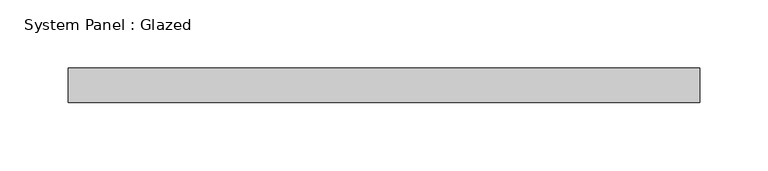
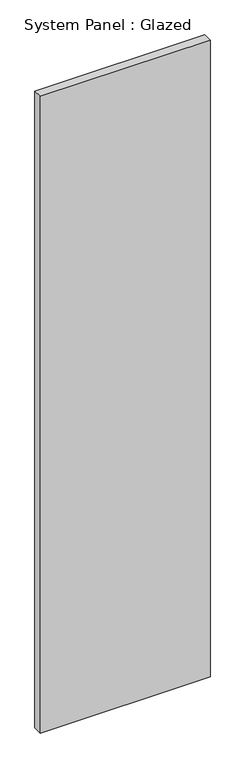
"""IFC4 building model written with IfcOpenShell, lengths in millimetres: plate geometry, System Panel : Glazed."""

from ifc_helpers import new_model, si_unit, origin, origin_with_axes, place, context, project, spatial, polyline, outline, extrude, source, transform, mapped, element, save


def system_panel_glazed_2a40583e(model_context):
    return source(origin(), model_context, "Body", "SweptSolid", [
        extrude(outline(polyline([(231.775, 19.05), (-231.775, 19.05), (-231.775, 44.45), (231.775, 44.45), (231.775, 19.05)])), origin_with_axes(), (0.0, 0.0, 1.0), 1837.4891744),
    ])


if __name__ == "__main__":
    model = new_model("IFC4")
    model_context = context("Model", 3, world=origin())
    ifc_project = project(units=[si_unit("LENGTHUNIT", "METRE", prefix="MILLI")], contexts=[model_context])
    site = spatial("IfcSite", under=ifc_project)
    building = spatial("IfcBuilding", under=site)
    placement = place(None, origin())
    system_panel_glazed_shape = system_panel_glazed_2a40583e(model_context)
    element("IfcPlate", 1, ObjectType="System Panel : Glazed", at=placement, inside=building, context=model_context, shape_type="MappedRepresentation", body=[
        mapped(system_panel_glazed_shape, transform((0.0, 0.0, 0.0), x_axis=(1.0, 0.0, 0.0), y_axis=(0.0, 1.0, 0.0), z_axis=(0.0, 0.0, 1.0))),
    ])
    save(model, "model.ifc")

# Revit data of these elements
# Type "System Panel : Glazed"
#   Construction Type Id = "GSP4R"
#   Analytic Construction = "1/8 in Pilkington single glazing"
#   Visual Light Transmittance = 0.9
#   Solar Heat Gain Coefficient = 0.86
#   Heat Transfer Coefficient (U) = 1.18115 BTU/(h·ft²·°F)
#   Define Thermal Properties by = 1
# Element 1 (IfcPlate, "System Panel : Glazed")
#   Materials on its faces: "Glass"
# Materials
#   "Glass": class "Glass", colour RGB 0 128 192, transparency 0.75, Description = "Soda Lime Glass", Cost = 0
